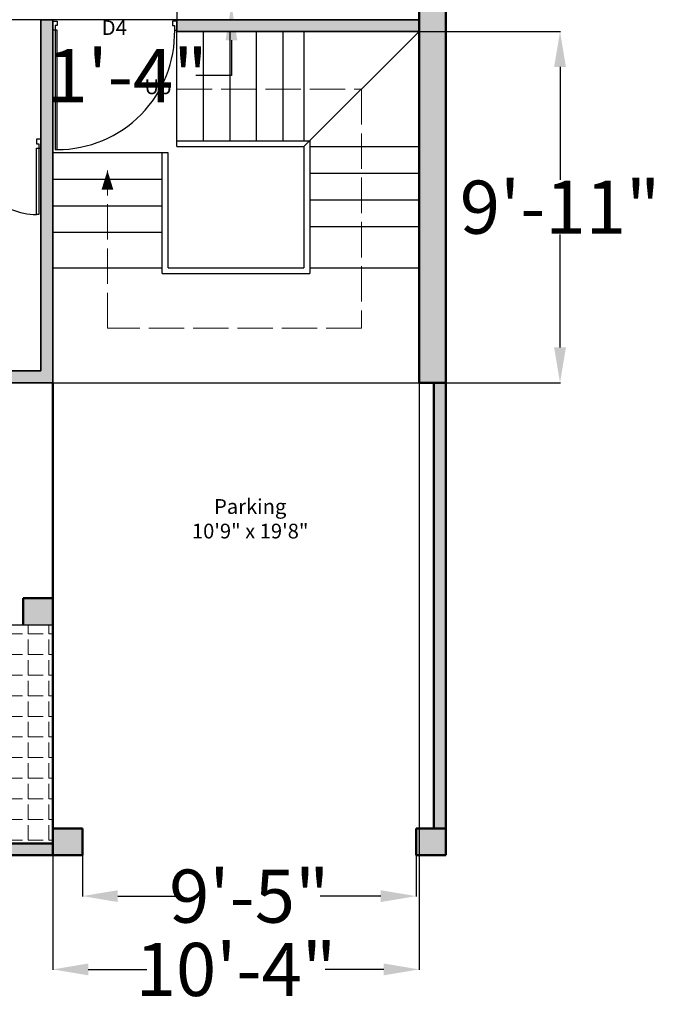
# Model space of a CAD drawing. Units: inches. Extents: x 2796 to 3603, y 978 to 1787.
# Tile 6 of 15: x 3280 to 3497, y 978 to 1312. Entities that reach past the tile are written whole.
import ezdxf

# ---------------------------------------------------------------- set-up
doc = ezdxf.new("R2010")
doc.units = ezdxf.units.IN
doc.linetypes.add('ACAD_ISO02W100', pattern=[15, 12, -3])
for name, color, linetype, lineweight in [('A-ANNO-DIMS', 7, 'Continuous', 18), ('A-ANNO-TEXT', 7, 'Continuous', 18), ('A-AREA-IDEN', 7, 'Continuous', 18), ('A-DOOR', 6, 'Continuous', 25), ('A-FLOR-STRS-PATH', 7, 'ACAD_ISO02W100', 13), ('A-WALL-EXTR-PATT', 1, 'Continuous', 13), ('A-WALL-INTR-PATT', 5, 'Continuous', 13), ('Inner Wall', 5, 'Continuous', 35), ('Kitchen', 3, 'Continuous', 25), ('L-PAVE', 1, 'Continuous', 25), ('L-PAVE-PATT', 7, 'Continuous', 13), ('Outer Wall', 1, 'Continuous', 50), ('Stairs', 8, 'Continuous', 25)]:
    doc.layers.add(name, color=color, linetype=linetype, lineweight=lineweight)
doc.styles.get("Standard").update_dxf_attribs({"font": 'arial.ttf'})
doc.dimstyles.get("Standard").update_dxf_attribs({"dimtxt": 18, "dimasz": 12, "dimexe": 0.18, "dimexo": 0.0625, "dimgap": 0.09, "dimtad": 0, "dimtih": 1, "dimtoh": 1, "dimdec": 0, "dimzin": 0, "dimdsep": 46, "dimlunit": 3, "dimtxsty": 'Standard', "dimcen": 0.09, "dimadec": 0, "dimazin": 0, "dimtfac": 1, "dimtdec": 0, "dimtofl": 0, "dimtmove": 0, "dimatfit": 3, "dimfxl": 1, "dimtolj": 1, "dimtzin": 0, "dimarcsym": 0})

# ---------------------------------------------------------------- blocks, each defined once
blk = doc.blocks.new('*D14')
at = {"layer": 'A-ANNO-DIMS', "color": 0, "lineweight": -2, "transparency": 16777216}
for p, q in [((3301.25, 1028.61), (3301.25, 1014.63)), ((3414.25, 1028.61), (3414.25, 1014.63)), ((3313.25, 1014.81), (3333.73, 1014.81)), ((3402.25, 1014.81), (3381.76, 1014.81))]:
    blk.add_line(p, q, dxfattribs=at)
at = {"layer": 'A-ANNO-DIMS', "color": 0, "transparency": 16777216}
for points in [[(3313.25, 1016.81), (3313.25, 1012.81), (3301.25, 1014.81)], [(3402.25, 1016.81), (3402.25, 1012.81), (3414.25, 1014.81)]]:
    blk.add_solid(points, dxfattribs=at)
at = {"layer": 'Defpoints', "color": 0, "transparency": 16777216}
for p in [(3301.25, 1028.68), (3414.25, 1028.68), (3414.25, 1014.81)]:
    blk.add_point(p, dxfattribs=at)
at = {"layer": 'A-ANNO-DIMS', "color": 0, "transparency": 16777216, "insert": (3357.75, 1014.81), "char_height": 18, "attachment_point": 5}
blk.add_mtext('\\A1;9\'-5"', dxfattribs=at)
blk = doc.blocks.new('DOOR-SWING-24IN')
for points in [[(-0.75, -0.7375), (-0.75, 21.7625), (0, 21.7625), (0, -0.7375)], [(-1.5, -3.7375), (0, -3.7375), (0, -2.2375), (-0.75, -2.2375), (-0.75, -0.7375), (-1.5, -0.7375)], [(22.5, -3.7375), (21, -3.7375), (21, -2.2375), (21.75, -2.2375), (21.75, -0.7375), (22.5, -0.7375)]]:
    blk.add_lwpolyline(points, close=True)
blk.add_arc((0, 0), 21.7625, 358.057956, 90)
blk = doc.blocks.new('*D34')
at = {"layer": 'A-ANNO-DIMS', "color": 0, "lineweight": -2, "transparency": 16777216}
for p, q in [((3355.83, 1336.87), (3343.83, 1336.87)), ((3355.83, 1332.81), (3355.83, 1337.05)), ((3371.32, 1336.87), (3367.83, 1336.87)), ((3383.32, 1332.81), (3383.32, 1337.05))]:
    blk.add_line(p, q, dxfattribs=at)
at = {"layer": 'A-ANNO-DIMS', "color": 0, "transparency": 16777216}
for points in [[(3367.83, 1338.87), (3367.83, 1334.87), (3355.83, 1336.87)], [(3371.32, 1338.87), (3371.32, 1334.87), (3383.32, 1336.87)]]:
    blk.add_solid(points, dxfattribs=at)
at = {"layer": 'Defpoints', "color": 0, "transparency": 16777216}
for p in [(3355.83, 1336.87), (3355.83, 1332.75), (3383.32, 1332.75)]:
    blk.add_point(p, dxfattribs=at)
at = {"layer": 'A-ANNO-DIMS', "color": 0, "transparency": 16777216, "insert": (3268.59, 1336.87), "char_height": 18, "attachment_point": 5}
blk.add_mtext('\\A1;HOB 2\'-3 1/2"', dxfattribs=at)
blk = doc.blocks.new('*D35')
at = {"layer": 'A-ANNO-DIMS', "color": 0, "lineweight": -2, "transparency": 16777216}
for p, q in [((3351.71, 1344.75), (3351.71, 1356.75)), ((3355.77, 1332.75), (3351.53, 1332.75)), ((3355.77, 1316.72), (3351.53, 1316.72)), ((3351.71, 1304.72), (3351.71, 1292.72)), ((3351.71, 1292.72), (3339.71, 1292.72))]:
    blk.add_line(p, q, dxfattribs=at)
at = {"layer": 'A-ANNO-DIMS', "color": 0, "transparency": 16777216}
for points in [[(3349.71, 1344.75), (3353.71, 1344.75), (3351.71, 1332.75)], [(3349.71, 1304.72), (3353.71, 1304.72), (3351.71, 1316.72)]]:
    blk.add_solid(points, dxfattribs=at)
at = {"layer": 'Defpoints', "color": 0, "transparency": 16777216}
for p in [(3355.83, 1332.75), (3351.71, 1316.72), (3355.83, 1316.72)]:
    blk.add_point(p, dxfattribs=at)
at = {"layer": 'A-ANNO-DIMS', "color": 0, "transparency": 16777216, "insert": (3316.54, 1292.72), "char_height": 18, "attachment_point": 5}
blk.add_mtext('\\A1;1\'-4"', dxfattribs=at)
blk = doc.blocks.new('*D43')
at = {"layer": 'A-ANNO-DIMS', "color": 0, "lineweight": -2, "transparency": 16777216}
for p, q in [((3291.25, 1188.61), (3291.25, 989.8)), ((3415.25, 1188.61), (3415.25, 989.8)), ((3303.25, 989.98), (3323.09, 989.98)), ((3403.25, 989.98), (3383.41, 989.98))]:
    blk.add_line(p, q, dxfattribs=at)
at = {"layer": 'A-ANNO-DIMS', "color": 0, "transparency": 16777216}
for points in [[(3303.25, 991.98), (3303.25, 987.98), (3291.25, 989.98)], [(3403.25, 991.98), (3403.25, 987.98), (3415.25, 989.98)]]:
    blk.add_solid(points, dxfattribs=at)
at = {"layer": 'Defpoints', "color": 0, "transparency": 16777216}
for p in [(3291.25, 1188.68), (3415.25, 1188.68), (3415.25, 989.98)]:
    blk.add_point(p, dxfattribs=at)
at = {"layer": 'A-ANNO-DIMS', "color": 0, "transparency": 16777216, "insert": (3353.25, 989.98), "char_height": 18, "attachment_point": 5}
blk.add_mtext('\\A1;10\'-4"', dxfattribs=at)
blk = doc.blocks.new('*D44')
at = {"layer": 'A-ANNO-DIMS', "color": 0, "lineweight": -2, "transparency": 16777216}
for p, q in [((3415.31, 1307.68), (3463.13, 1307.68)), ((3462.95, 1295.68), (3462.95, 1257.46)), ((3462.95, 1200.68), (3462.95, 1238.9)), ((3415.31, 1188.68), (3463.13, 1188.68))]:
    blk.add_line(p, q, dxfattribs=at)
at = {"layer": 'A-ANNO-DIMS', "color": 0, "transparency": 16777216}
for points in [[(3460.95, 1295.68), (3464.95, 1295.68), (3462.95, 1307.68)], [(3460.95, 1200.68), (3464.95, 1200.68), (3462.95, 1188.68)]]:
    blk.add_solid(points, dxfattribs=at)
at = {"layer": 'Defpoints', "color": 0, "transparency": 16777216}
for p in [(3415.25, 1307.68), (3462.95, 1307.68), (3415.25, 1188.68)]:
    blk.add_point(p, dxfattribs=at)
at = {"layer": 'A-ANNO-DIMS', "color": 0, "transparency": 16777216, "insert": (3462.95, 1248.18), "char_height": 18, "attachment_point": 5}
blk.add_mtext('\\A1;9\'-11"', dxfattribs=at)
blk = doc.blocks.new('*D53')
at = {"layer": 'A-ANNO-DIMS', "color": 0, "lineweight": -2, "transparency": 16777216}
for p, q in [((3031.545499, 1347.67534), (3031.545499, 1359.67534)), ((3333.182999, 1335.67534), (3031.365499, 1335.67534)), ((3333.182999, 1311.67534), (3031.365499, 1311.67534)), ((3031.545499, 1299.67534), (3031.545499, 1287.67534))]:
    blk.add_line(p, q, dxfattribs=at)
at = {"layer": 'A-ANNO-DIMS', "color": 0, "transparency": 16777216}
for points in [[(3029.545499, 1347.67534), (3033.545499, 1347.67534), (3031.545499, 1335.67534)], [(3029.545499, 1299.67534), (3033.545499, 1299.67534), (3031.545499, 1311.67534)]]:
    blk.add_solid(points, dxfattribs=at)
at = {"layer": 'Defpoints', "color": 0, "transparency": 16777216}
for p in [(3031.545499, 1335.67534), (3333.245499, 1335.67534), (3333.245499, 1311.67534)]:
    blk.add_point(p, dxfattribs=at)
at = {"layer": 'A-ANNO-DIMS', "color": 0, "transparency": 16777216, "insert": (3031.545499, 1323.67534), "char_height": 18, "attachment_point": 5}
blk.add_mtext('\\A1;2\'-0"', dxfattribs=at)

msp = doc.modelspace()

# ---------------------------------------------------------------- hatches: boundary and pattern name
at = {"layer": 'A-WALL-EXTR-PATT'}
h = msp.add_hatch(color=256, dxfattribs=at)
h.dxf.hatch_style = 1
h.paths.add_polyline_path([(3424.25, 1736.68), (3070.25, 1736.68), (3070.25, 1106.68), (3227.25, 1106.68), (3227.25, 1115.68), (3226.75, 1115.68), (3223.75, 1115.68), (3079.25, 1115.68), (3079.25, 1727.68), (3127.25, 1727.68), (3415.25, 1727.68), (3415.25, 1188.68), (3424.25, 1188.68)])
h.paths.add_polyline_path([(3291.25, 1032.68), (3074.25, 1032.68), (3074.25, 1106.68), (3070.25, 1106.68), (3070.25, 1028.68), (3291.25, 1028.68)])
h.paths.add_polyline_path([(3291.25, 1115.68), (3281.25, 1115.68), (3281.25, 1106.68), (3291.25, 1106.68)], flags=17)
h.paths.add_polyline_path([(3301.25, 1037.68), (3291.25, 1037.68), (3291.25, 1028.68), (3301.25, 1028.68)])
h.paths.add_polyline_path([(3424.25, 1037.68), (3414.25, 1037.68), (3414.25, 1028.68), (3424.25, 1028.68)])
h.paths.add_polyline_path([(3424.25, 1188.68), (3420.25, 1188.68), (3420.25, 1037.68), (3424.25, 1037.68)])
at = {"layer": 'A-WALL-INTR-PATT'}
h = msp.add_hatch(color=256, dxfattribs=at)
h.dxf.hatch_style = 1
h.paths.add_polyline_path([(3249.25, 1727.68), (3245.25, 1727.68), (3245.25, 1655.68), (3103.25, 1655.68), (3103.25, 1651.68), (3245.25, 1651.68), (3245.25, 1503.68), (3249.25, 1503.68)])
h.paths.add_polyline_path([(3131.25, 1727.68), (3127.25, 1727.68), (3127.25, 1703.68), (3127.25, 1679.68), (3131.25, 1679.68)], flags=17)
h.paths.add_polyline_path([(3391.25, 1655.68), (3325.25, 1655.68), (3325.25, 1727.68), (3321.25, 1727.68), (3321.25, 1655.68), (3273.25, 1655.68), (3273.25, 1651.68), (3391.25, 1651.68)])
h.paths.add_polyline_path([(3203.25, 1459.68), (3079.25, 1459.68), (3079.25, 1455.68), (3199.25, 1455.68), (3199.25, 1431.68), (3199.25, 1347.68), (3203.25, 1347.68)])
h.paths.add_polyline_path([(3209.25, 1507.68), (3079.25, 1507.68), (3079.25, 1503.68), (3209.25, 1503.68)])
h.paths.add_polyline_path([(3415.25, 1507.68), (3285.25, 1507.68), (3285.25, 1503.68), (3415.25, 1503.68)])
h.paths.add_polyline_path([(3415.25, 1459.68), (3333.25, 1459.68), (3333.25, 1455.68), (3415.25, 1455.68)])
h.paths.add_polyline_path([(3291.25, 1311.68), (3287.25, 1311.68), (3287.25, 1192.68), (3227.25, 1192.68), (3227.25, 1267.68), (3263.25, 1267.68), (3263.25, 1271.68), (3223.25, 1271.68), (3223.25, 1151.68), (3227.25, 1151.68), (3227.25, 1188.68), (3291.25, 1188.68)])
h.paths.add_polyline_path([(3227.25, 1311.68), (3079.25, 1311.68), (3079.25, 1307.68), (3227.25, 1307.68)])
h = msp.add_hatch(color=256, dxfattribs=at)
h.dxf.hatch_style = 1
h.paths.add_polyline_path([(3415.25, 1311.68), (3333.25, 1311.68), (3333.25, 1307.68), (3415.25, 1307.68)])
at = {"layer": 'L-PAVE-PATT'}
h = msp.add_hatch(dxfattribs=at)
h.set_pattern_fill('ANGLE', color=256)
h.set_pattern_definition([(0, (0, 0), (0, 6.985), [5.08, -1.905]), (90, (0, 0), (-6.985, 4e-16), [5.08, -1.905])])
h.paths.add_polyline_path([(3291.25, 1106.68), (3227.25, 1106.68), (3227.25, 1032.68), (3291.25, 1032.68)])

# ---------------------------------------------------------------- linework, layer by layer
at = {"layer": 'A-DOOR'}
for points in [[(3291.25, 1311.18), (3292.75, 1311.18), (3292.75, 1309.68), (3292, 1309.68), (3292, 1308.18), (3291.25, 1308.18)], [(3333.25, 1311.18), (3331.75, 1311.18), (3331.75, 1309.68), (3332.5, 1309.68), (3332.5, 1308.18), (3333.25, 1308.18)], [(3292, 1308.18), (3292, 1267.68), (3292.75, 1267.68), (3292.75, 1308.18)]]:
    msp.add_lwpolyline(points, close=True, dxfattribs=at)
msp.add_arc((3292.75, 1307.43), 39.76, 270, 1.0709, dxfattribs=at)
at = {"layer": 'A-FLOR-STRS-PATH'}
for p, q in [((3333.25, 1288.18), (3395.75, 1288.18)), ((3395.75, 1288.18), (3395.75, 1207.18)), ((3309.75, 1207.18), (3309.75, 1260.62)), ((3395.75, 1207.18), (3309.75, 1207.18))]:
    msp.add_line(p, q, dxfattribs=at)
at = {"layer": 'Inner Wall'}
for p, q in [((3287.25, 1192.68), (3287.25, 1311.68)), ((3291.25, 1311.68), (3287.25, 1311.68)), ((3291.25, 1188.68), (3291.25, 1311.68)), ((3333.25, 1311.68), (3415.25, 1311.68)), ((3333.25, 1307.68), (3333.25, 1311.68)), ((3333.25, 1307.68), (3415.25, 1307.68)), ((3227.25, 1192.68), (3287.25, 1192.68)), ((3227.25, 1188.68), (3291.25, 1188.68))]:
    msp.add_line(p, q, dxfattribs=at)
at = {"layer": 'Kitchen'}
for p, q in [((3415.25, 1455.68), (3415.25, 1311.68)), ((3333.25, 1335.68), (3333.25, 1311.68)), ((3415.25, 1311.68), (3333.25, 1311.68))]:
    msp.add_line(p, q, dxfattribs=at)
at = {"layer": 'L-PAVE'}
msp.add_line((3227.25, 1106.68), (3291.25, 1106.68), dxfattribs=at)
at = {"layer": 'Outer Wall'}
for p, q in [((3424.25, 1736.68), (3424.25, 1028.68)), ((3415.25, 1727.68), (3415.25, 1188.68)), ((3291.25, 1028.68), (3291.25, 1188.68)), ((3415.25, 1188.68), (3424.25, 1188.68)), ((3420.25, 1188.68), (3420.25, 1037.68)), ((3281.25, 1106.68), (3281.25, 1115.68)), ((3281.25, 1115.68), (3291.25, 1115.68)), ((3291.25, 1037.68), (3301.25, 1037.68)), ((3301.25, 1028.68), (3301.25, 1037.68)), ((3414.25, 1037.68), (3424.25, 1037.68)), ((3414.25, 1028.68), (3414.25, 1037.68)), ((3070.25, 1028.68), (3301.25, 1028.68)), ((3414.25, 1028.68), (3424.25, 1028.68)), ((3424.25, 1028.68), (3414.25, 1028.68))]:
    msp.add_line(p, q, dxfattribs=at)
msp.add_lwpolyline([(3291.25, 1032.68), (3074.25, 1032.68), (3074.25, 1106.68)], dxfattribs=at)
at = {"layer": 'Stairs'}
for p, q in [((3333.25, 1268.68), (3333.25, 1307.68)), ((3342.25, 1270.68), (3342.25, 1307.68)), ((3351.25, 1270.68), (3351.25, 1307.68)), ((3360.25, 1270.68), (3360.25, 1307.68)), ((3369.25, 1270.68), (3369.25, 1307.68)), ((3376.25, 1307.68), (3376.25, 1270.68)), ((3376.25, 1268.68), (3415.25, 1307.68)), ((3333.25, 1270.68), (3378.25, 1270.68)), ((3333.25, 1268.68), (3376.25, 1268.68)), ((3376.25, 1268.68), (3376.25, 1227.68)), ((3378.25, 1270.68), (3378.25, 1225.68)), ((3378.25, 1268.68), (3415.25, 1268.68)), ((3330.25, 1266.54), (3291.25, 1266.54)), ((3328.25, 1225.68), (3328.25, 1266.54)), ((3330.25, 1227.68), (3330.25, 1266.54)), ((3328.25, 1257.54), (3291.25, 1257.54)), ((3378.25, 1259.68), (3415.25, 1259.68)), ((3378.25, 1250.68), (3415.25, 1250.68)), ((3328.25, 1248.54), (3291.25, 1248.54)), ((3378.25, 1241.68), (3415.25, 1241.68)), ((3328.25, 1239.54), (3291.25, 1239.54)), ((3291.25, 1227.68), (3328.25, 1227.68)), ((3330.25, 1227.68), (3376.25, 1227.68)), ((3378.25, 1227.68), (3415.25, 1227.68)), ((3328.25, 1225.68), (3378.25, 1225.68)), ((3291.25, 1188.68), (3415.25, 1188.68))]:
    msp.add_line(p, q, dxfattribs=at)
msp.add_lwpolyline([(3309.75, 1260.62, 0, 4, 0), (3309.75, 1254.06, 4, 4, 0)], format="xyseb", dxfattribs=at)

# ---------------------------------------------------------------- block references
at = {"layer": 'A-DOOR', "rotation": 180}
msp.add_blockref('DOOR-SWING-24IN', (3285.75, 1267.44), dxfattribs=at)

# ---------------------------------------------------------------- texts
at = {"layer": 'A-ANNO-TEXT', "char_height": 5, "attachment_point": 3}
for s, insert in [('\\pxqc;{\\fTimes New Roman|b0|i0|c0|p18;D4}', (3319.91, 1311.48)), ('\\pxqc;{\\fTimes New Roman|b0|i0|c0|p18;Up}', (3334.7, 1291.46))]:
    msp.add_mtext_dynamic_manual_height_columns(s, width=15.6741, gutter_width=12.5, heights=[0], dxfattribs=dict(at, insert=insert))
at = {"layer": 'A-AREA-IDEN', "insert": (3385.82, 1149.29), "char_height": 5, "attachment_point": 3}
msp.add_mtext_dynamic_manual_height_columns('\\pxqc;{\\fTimes New Roman|b0|i0|c0|p18;Parking\\P10\'9" x 19\'8"}', width=55.5021, gutter_width=12.5, heights=[0], dxfattribs=at)

# ---------------------------------------------------------------- dimensions: what is measured, and where the dimension line sits
at = {"layer": 'A-ANNO-DIMS'}
dim = msp.add_linear_dim(base=(3355.83, 1336.87), p1=(3383.32, 1332.75), p2=(3355.83, 1332.75), angle=180, text='HOB <>', dimstyle='Standard', override={"dimdec": 1, "dimlfac": 1, "dimrnd": 0, "dimzin": 1, "dimdsep": 46, "dimlunit": 4, "dimfrac": 2}, dxfattribs=at)
dim.commit()
dim.dimension.update_dxf_attribs({"geometry": '*D34', "text_midpoint": (3268.59, 1336.87)})
for base, p1, p2, angle, picture, middle in [((3031.55, 1335.68), (3333.25, 1311.68), (3333.25, 1335.68), 90, '*D53', (3031.55, 1323.68)), ((3351.71, 1316.72), (3355.83, 1332.75), (3355.83, 1316.72), 270, '*D35', (3316.54, 1292.72)), ((3462.95, 1307.68), (3415.25, 1188.68), (3415.25, 1307.68), 90, '*D44', (3462.95, 1248.18))]:
    dim = msp.add_linear_dim(base=base, p1=p1, p2=p2, angle=angle, dimstyle='Standard', override={"dimdec": 1, "dimlfac": 1, "dimrnd": 0, "dimzin": 1, "dimdsep": 46, "dimlunit": 4, "dimfrac": 2}, dxfattribs=at)
    dim.commit()
    dim.dimension.update_dxf_attribs({"geometry": picture, "text_midpoint": middle})
for base, p1, p2, override, picture, middle in [((3415.25, 989.98), (3291.25, 1188.68), (3415.25, 1188.68), {"dimdec": 1, "dimlfac": 1, "dimrnd": 0, "dimzin": 1, "dimdsep": 46, "dimlunit": 4, "dimfrac": 2}, '*D43', (3353.25, 989.98)), ((3414.25, 1014.81), (3301.25, 1028.68), (3414.25, 1028.68), {"dimclrd": 0, "dimclre": 0, "dimclrt": 0}, '*D14', (3357.75, 1014.81))]:
    dim = msp.add_linear_dim(base=base, p1=p1, p2=p2, dimstyle='Standard', override=override, dxfattribs=at)
    dim.commit()
    dim.dimension.update_dxf_attribs({"geometry": picture, "text_midpoint": middle})

doc.saveas('drawing.dxf')
